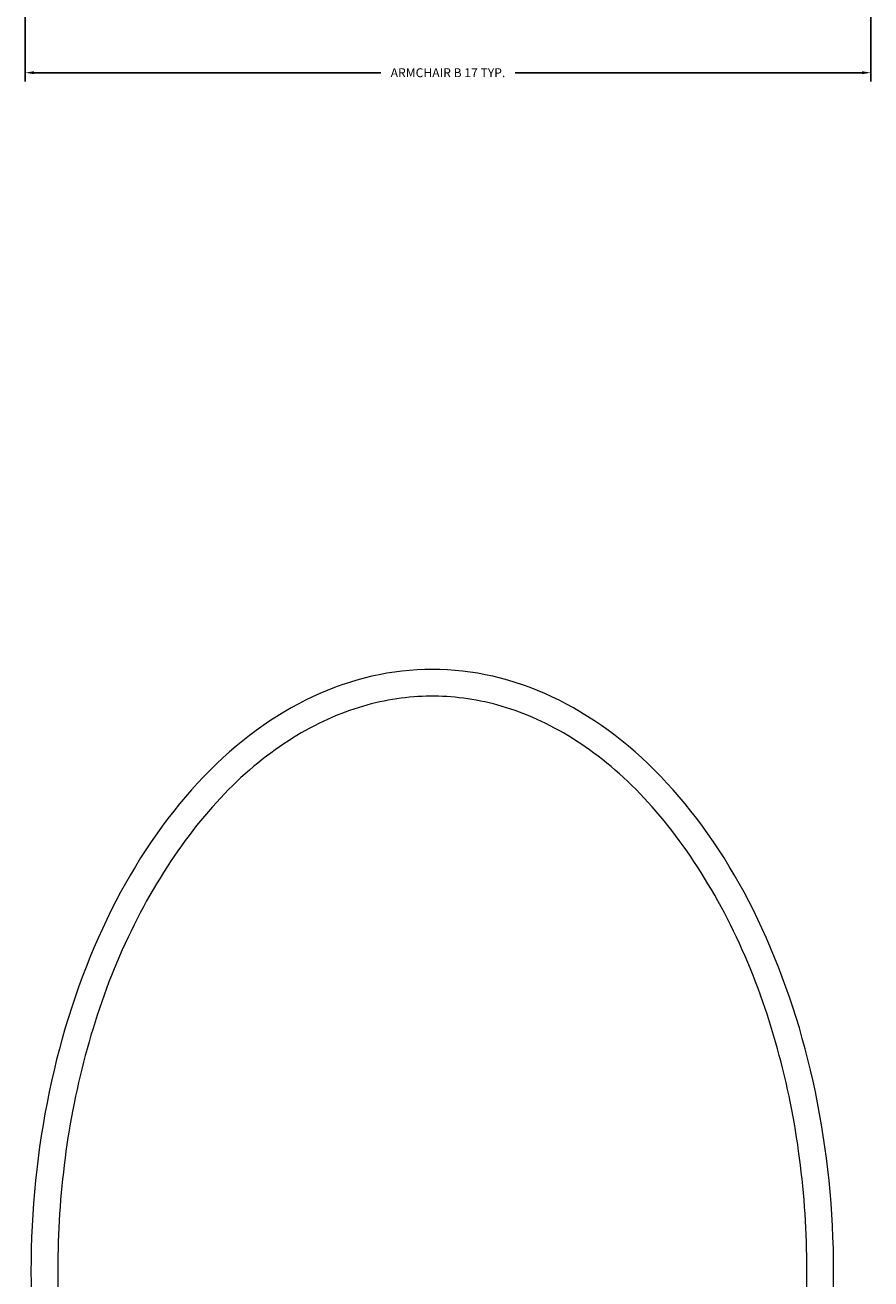
# Model space of a CAD drawing. Units: inches. Extents: x 963 to 2075, y 289 to 2657.
# Tile 75 of 98: x 1467 to 1485, y 2265 to 2290. Entities that reach past the tile are written whole.
import ezdxf

# ---------------------------------------------------------------- set-up
doc = ezdxf.new("R2010")
doc.units = ezdxf.units.IN
doc.layers.add('A-ANNO-DIMS', color=2, linetype='Continuous', lineweight=18)
doc.layers.add('A-FURN', color=8, linetype='Continuous', lineweight=18)
doc.styles.get("Standard").update_dxf_attribs({"font": 'arial.ttf'})
doc.dimstyles.get("Standard").update_dxf_attribs({"dimtxt": 0.18, "dimasz": 0.18, "dimexe": 0.18, "dimexo": 0.0625, "dimgap": 0.09, "dimtad": 0, "dimtih": 1, "dimtoh": 1, "dimdec": 4, "dimzin": 0, "dimdsep": 46, "dimtxsty": 'Standard', "dimcen": 0.09, "dimadec": 0, "dimazin": 0, "dimtfac": 1, "dimtdec": 4, "dimtofl": 0, "dimtmove": 0, "dimatfit": 3, "dimfxl": 1, "dimtolj": 1, "dimtzin": 0, "dimarcsym": 0})

# ---------------------------------------------------------------- blocks, each defined once
blk = doc.blocks.new('TABLE-OVAL')
at = {"ltscale": 0.03}
blk.add_polyline3d([(7.656, -0.197, 0), (7.809, -0.194, 0), (7.963, -0.188, 0), (8.116, -0.177, 0), (8.269, -0.162, 0), (8.422, -0.142, 0), (8.575, -0.118, 0), (8.727, -0.09, 0), (8.879, -0.057, 0), (9.031, -0.021, 0), (9.182, 0.021, 0), (9.332, 0.066, 0), (9.482, 0.116, 0), (9.632, 0.17, 0), (9.78, 0.228, 0), (9.928, 0.29, 0), (10.075, 0.357, 0), (10.221, 0.428, 0), (10.366, 0.503, 0), (10.51, 0.582, 0), (10.653, 0.665, 0), (10.796, 0.752, 0), (10.937, 0.843, 0), (11.076, 0.938, 0), (11.215, 1.037, 0), (11.352, 1.14, 0), (11.488, 1.247, 0), (11.623, 1.358, 0), (11.756, 1.472, 0), (11.888, 1.59, 0), (12.018, 1.712, 0), (12.147, 1.838, 0), (12.274, 1.967, 0), (12.399, 2.1, 0), (12.523, 2.237, 0), (12.645, 2.376, 0), (12.765, 2.52, 0), (12.883, 2.666, 0), (13, 2.817, 0), (13.114, 2.97, 0), (13.227, 3.126, 0), (13.337, 3.286, 0), (13.446, 3.449, 0), (13.552, 3.615, 0), (13.657, 3.784, 0), (13.759, 3.955, 0), (13.859, 4.13, 0), (13.957, 4.308, 0), (14.052, 4.488, 0), (14.145, 4.671, 0), (14.236, 4.856, 0), (14.325, 5.044, 0), (14.411, 5.235, 0), (14.495, 5.428, 0), (14.576, 5.623, 0), (14.655, 5.821, 0), (14.731, 6.021, 0), (14.805, 6.222, 0), (14.877, 6.426, 0), (14.945, 6.632, 0), (15.011, 6.84, 0), (15.075, 7.05, 0), (15.135, 7.261, 0), (15.193, 7.475, 0), (15.249, 7.689, 0), (15.301, 7.906, 0), (15.351, 8.123, 0), (15.399, 8.343, 0), (15.443, 8.563, 0), (15.485, 8.785, 0), (15.523, 9.007, 0), (15.559, 9.231, 0), (15.592, 9.456, 0), (15.623, 9.682, 0), (15.65, 9.908, 0), (15.675, 10.136, 0), (15.697, 10.364, 0), (15.715, 10.592, 0), (15.731, 10.821, 0), (15.744, 11.051, 0), (15.755, 11.28, 0), (15.762, 11.51, 0), (15.766, 11.741, 0), (15.768, 11.971, 0), (15.766, 12.201, 0), (15.762, 12.431, 0), (15.755, 12.661, 0), (15.744, 12.891, 0), (15.731, 13.12, 0), (15.715, 13.349, 0), (15.697, 13.578, 0), (15.675, 13.806, 0), (15.65, 14.033, 0), (15.623, 14.26, 0), (15.592, 14.486, 0), (15.559, 14.71, 0), (15.523, 14.934, 0), (15.485, 15.157, 0), (15.443, 15.379, 0), (15.399, 15.599, 0), (15.351, 15.818, 0), (15.301, 16.036, 0), (15.249, 16.252, 0), (15.193, 16.467, 0), (15.135, 16.68, 0), (15.075, 16.892, 0), (15.011, 17.101, 0), (14.945, 17.309, 0), (14.877, 17.515, 0), (14.805, 17.719, 0), (14.731, 17.921, 0), (14.655, 18.121, 0), (14.576, 18.318, 0), (14.495, 18.514, 0), (14.411, 18.707, 0), (14.325, 18.897, 0), (14.236, 19.085, 0), (14.145, 19.271, 0), (14.052, 19.454, 0), (13.957, 19.634, 0), (13.859, 19.811, 0), (13.759, 19.986, 0), (13.657, 20.158, 0), (13.552, 20.327, 0), (13.446, 20.493, 0), (13.337, 20.656, 0), (13.227, 20.815, 0), (13.114, 20.972, 0), (13, 21.125, 0), (12.883, 21.275, 0), (12.765, 21.422, 0), (12.645, 21.565, 0), (12.523, 21.705, 0), (12.399, 21.842, 0), (12.274, 21.974, 0), (12.147, 22.104, 0), (12.018, 22.229, 0), (11.888, 22.351, 0), (11.756, 22.47, 0), (11.623, 22.584, 0), (11.488, 22.695, 0), (11.352, 22.802, 0), (11.215, 22.905, 0), (11.076, 23.004, 0), (10.937, 23.099, 0), (10.796, 23.19, 0), (10.653, 23.277, 0), (10.51, 23.36, 0), (10.366, 23.439, 0), (10.221, 23.514, 0), (10.075, 23.585, 0), (9.928, 23.651, 0), (9.78, 23.714, 0), (9.632, 23.772, 0), (9.482, 23.826, 0), (9.332, 23.876, 0), (9.182, 23.921, 0), (9.031, 23.962, 0), (8.879, 23.999, 0), (8.727, 24.032, 0), (8.575, 24.06, 0), (8.422, 24.084, 0), (8.269, 24.103, 0), (8.116, 24.119, 0), (7.963, 24.13, 0), (7.809, 24.136, 0), (7.656, 24.138, 0), (7.502, 24.136, 0), (7.349, 24.13, 0), (7.196, 24.119, 0), (7.042, 24.103, 0), (6.89, 24.084, 0), (6.737, 24.06, 0), (6.585, 24.032, 0), (6.433, 23.999, 0), (6.281, 23.962, 0), (6.13, 23.921, 0), (5.979, 23.876, 0), (5.83, 23.826, 0), (5.68, 23.772, 0), (5.532, 23.714, 0), (5.384, 23.651, 0), (5.237, 23.585, 0), (5.091, 23.514, 0), (4.946, 23.439, 0), (4.802, 23.36, 0), (4.658, 23.277, 0), (4.516, 23.19, 0), (4.375, 23.099, 0), (4.236, 23.004, 0), (4.097, 22.905, 0), (3.96, 22.802, 0), (3.824, 22.695, 0), (3.689, 22.584, 0), (3.556, 22.47, 0), (3.424, 22.351, 0), (3.294, 22.229, 0), (3.165, 22.104, 0), (3.038, 21.974, 0), (2.913, 21.842, 0), (2.789, 21.705, 0), (2.667, 21.565, 0), (2.547, 21.422, 0), (2.429, 21.275, 0), (2.312, 21.125, 0), (2.198, 20.972, 0), (2.085, 20.815, 0), (1.975, 20.656, 0), (1.866, 20.493, 0), (1.76, 20.327, 0), (1.655, 20.158, 0), (1.553, 19.986, 0), (1.453, 19.811, 0), (1.355, 19.634, 0), (1.26, 19.454, 0), (1.166, 19.271, 0), (1.076, 19.085, 0), (0.987, 18.897, 0), (0.901, 18.707, 0), (0.817, 18.514, 0), (0.736, 18.318, 0), (0.657, 18.121, 0), (0.58, 17.921, 0), (0.507, 17.719, 0), (0.435, 17.515, 0), (0.367, 17.309, 0), (0.301, 17.101, 0), (0.237, 16.892, 0), (0.177, 16.68, 0), (0.118, 16.467, 0), (0.063, 16.252, 0), (0.01, 16.036, 0), (-0.039, 15.818, 0), (-0.087, 15.599, 0), (-0.131, 15.379, 0), (-0.173, 15.157, 0), (-0.211, 14.934, 0), (-0.247, 14.71, 0), (-0.281, 14.486, 0), (-0.311, 14.26, 0), (-0.338, 14.033, 0), (-0.363, 13.806, 0), (-0.385, 13.578, 0), (-0.403, 13.349, 0), (-0.419, 13.12, 0), (-0.432, 12.891, 0), (-0.443, 12.661, 0), (-0.45, 12.431, 0), (-0.454, 12.201, 0), (-0.456, 11.971, 0), (-0.454, 11.741, 0), (-0.45, 11.51, 0), (-0.443, 11.28, 0), (-0.432, 11.051, 0), (-0.419, 10.821, 0), (-0.403, 10.592, 0), (-0.385, 10.364, 0), (-0.363, 10.136, 0), (-0.338, 9.908, 0), (-0.311, 9.682, 0), (-0.281, 9.456, 0), (-0.247, 9.231, 0), (-0.211, 9.007, 0), (-0.173, 8.785, 0), (-0.131, 8.563, 0), (-0.087, 8.343, 0), (-0.039, 8.123, 0), (0.01, 7.906, 0), (0.063, 7.689, 0), (0.118, 7.475, 0), (0.177, 7.261, 0), (0.237, 7.05, 0), (0.301, 6.84, 0), (0.367, 6.632, 0), (0.435, 6.426, 0), (0.507, 6.222, 0), (0.58, 6.021, 0), (0.657, 5.821, 0), (0.736, 5.623, 0), (0.817, 5.428, 0), (0.901, 5.235, 0), (0.987, 5.044, 0), (1.076, 4.856, 0), (1.166, 4.671, 0), (1.26, 4.488, 0), (1.355, 4.308, 0), (1.453, 4.13, 0), (1.553, 3.955, 0), (1.655, 3.784, 0), (1.76, 3.615, 0), (1.866, 3.449, 0), (1.975, 3.286, 0), (2.085, 3.126, 0), (2.198, 2.97, 0), (2.312, 2.817, 0), (2.429, 2.666, 0), (2.547, 2.52, 0), (2.667, 2.376, 0), (2.789, 2.237, 0), (2.913, 2.1, 0), (3.038, 1.967, 0), (3.165, 1.838, 0), (3.294, 1.712, 0), (3.424, 1.59, 0), (3.556, 1.472, 0), (3.689, 1.358, 0), (3.824, 1.247, 0), (3.96, 1.14, 0), (4.097, 1.037, 0), (4.236, 0.938, 0), (4.375, 0.843, 0), (4.516, 0.752, 0), (4.658, 0.665, 0), (4.802, 0.582, 0), (4.946, 0.503, 0), (5.091, 0.428, 0), (5.237, 0.357, 0), (5.384, 0.29, 0), (5.532, 0.228, 0), (5.68, 0.17, 0), (5.83, 0.116, 0), (5.979, 0.066, 0), (6.13, 0.021, 0), (6.281, -0.021, 0), (6.433, -0.057, 0), (6.585, -0.09, 0), (6.737, -0.118, 0), (6.89, -0.142, 0), (7.042, -0.162, 0), (7.196, -0.177, 0), (7.349, -0.188, 0), (7.502, -0.194, 0), (7.656, -0.197, 0)], dxfattribs=at)
blk.add_polyline3d([(7.656, 0.344, 0), (7.739, 0.345, 0), (7.822, 0.347, 0), (7.906, 0.351, 0), (7.99, 0.356, 0), (8.074, 0.362, 0), (8.159, 0.37, 0), (8.244, 0.38, 0), (8.33, 0.391, 0), (8.415, 0.404, 0), (8.501, 0.418, 0), (8.588, 0.434, 0), (8.674, 0.451, 0), (8.761, 0.47, 0), (8.848, 0.491, 0), (8.935, 0.513, 0), (9.023, 0.538, 0), (9.11, 0.563, 0), (9.198, 0.591, 0), (9.286, 0.62, 0), (9.375, 0.651, 0), (9.463, 0.684, 0), (9.552, 0.719, 0), (9.64, 0.755, 0), (9.729, 0.794, 0), (9.818, 0.834, 0), (9.907, 0.876, 0), (9.995, 0.92, 0), (10.084, 0.966, 0), (10.173, 1.013, 0), (10.262, 1.063, 0), (10.35, 1.114, 0), (10.439, 1.167, 0), (10.527, 1.222, 0), (10.615, 1.279, 0), (10.703, 1.338, 0), (10.791, 1.398, 0), (10.878, 1.461, 0), (10.965, 1.525, 0), (11.052, 1.592, 0), (11.139, 1.66, 0), (11.225, 1.73, 0), (11.311, 1.802, 0), (11.396, 1.876, 0), (11.481, 1.952, 0), (11.565, 2.03, 0), (11.649, 2.109, 0), (11.733, 2.191, 0), (11.815, 2.275, 0), (11.898, 2.361, 0), (11.98, 2.448, 0), (12.061, 2.537, 0), (12.141, 2.629, 0), (12.221, 2.721, 0), (12.301, 2.816, 0), (12.379, 2.912, 0), (12.457, 3.01, 0), (12.535, 3.11, 0), (12.611, 3.211, 0), (12.687, 3.314, 0), (12.762, 3.418, 0), (12.836, 3.524, 0), (12.909, 3.632, 0), (12.982, 3.741, 0), (13.053, 3.851, 0), (13.124, 3.963, 0), (13.194, 4.076, 0), (13.262, 4.191, 0), (13.33, 4.307, 0), (13.397, 4.424, 0), (13.463, 4.543, 0), (13.528, 4.662, 0), (13.591, 4.783, 0), (13.654, 4.906, 0), (13.716, 5.029, 0), (13.776, 5.154, 0), (13.835, 5.279, 0), (13.893, 5.406, 0), (13.95, 5.534, 0), (14.006, 5.663, 0), (14.061, 5.792, 0), (14.114, 5.923, 0), (14.166, 6.055, 0), (14.217, 6.188, 0), (14.266, 6.321, 0), (14.314, 6.455, 0), (14.361, 6.589, 0), (14.406, 6.723, 0), (14.45, 6.858, 0), (14.493, 6.993, 0), (14.535, 7.129, 0), (14.575, 7.265, 0), (14.614, 7.401, 0), (14.652, 7.537, 0), (14.688, 7.674, 0), (14.724, 7.811, 0), (14.758, 7.948, 0), (14.791, 8.086, 0), (14.822, 8.223, 0), (14.852, 8.361, 0), (14.882, 8.5, 0), (14.909, 8.638, 0), (14.936, 8.777, 0), (14.961, 8.916, 0), (14.986, 9.055, 0), (15.009, 9.194, 0), (15.031, 9.334, 0), (15.051, 9.473, 0), (15.071, 9.613, 0), (15.089, 9.753, 0), (15.106, 9.893, 0), (15.122, 10.033, 0), (15.137, 10.174, 0), (15.151, 10.314, 0), (15.163, 10.455, 0), (15.175, 10.596, 0), (15.185, 10.736, 0), (15.194, 10.877, 0), (15.202, 11.018, 0), (15.209, 11.159, 0), (15.215, 11.3, 0), (15.219, 11.441, 0), (15.223, 11.583, 0), (15.225, 11.724, 0), (15.227, 11.865, 0), (15.227, 12.006, 0), (15.226, 12.147, 0), (15.224, 12.288, 0), (15.221, 12.43, 0), (15.217, 12.571, 0), (15.212, 12.712, 0), (15.205, 12.853, 0), (15.198, 12.994, 0), (15.19, 13.135, 0), (15.18, 13.276, 0), (15.169, 13.416, 0), (15.157, 13.557, 0), (15.144, 13.698, 0), (15.13, 13.838, 0), (15.114, 13.978, 0), (15.098, 14.119, 0), (15.08, 14.259, 0), (15.061, 14.399, 0), (15.041, 14.538, 0), (15.02, 14.678, 0), (14.997, 14.817, 0), (14.974, 14.956, 0), (14.949, 15.095, 0), (14.923, 15.234, 0), (14.896, 15.373, 0), (14.867, 15.511, 0), (14.837, 15.649, 0), (14.806, 15.787, 0), (14.774, 15.925, 0), (14.741, 16.062, 0), (14.706, 16.199, 0), (14.67, 16.336, 0), (14.633, 16.473, 0), (14.595, 16.609, 0), (14.555, 16.745, 0), (14.514, 16.881, 0), (14.472, 17.016, 0), (14.428, 17.151, 0), (14.384, 17.286, 0), (14.338, 17.42, 0), (14.29, 17.554, 0), (14.241, 17.687, 0), (14.191, 17.821, 0), (14.14, 17.953, 0), (14.087, 18.084, 0), (14.034, 18.214, 0), (13.978, 18.344, 0), (13.922, 18.472, 0), (13.865, 18.599, 0), (13.806, 18.725, 0), (13.746, 18.85, 0), (13.685, 18.974, 0), (13.623, 19.097, 0), (13.56, 19.219, 0), (13.495, 19.339, 0), (13.43, 19.458, 0), (13.364, 19.576, 0), (13.296, 19.693, 0), (13.228, 19.808, 0), (13.159, 19.922, 0), (13.089, 20.035, 0), (13.017, 20.146, 0), (12.945, 20.255, 0), (12.873, 20.364, 0), (12.799, 20.47, 0), (12.724, 20.576, 0), (12.649, 20.679, 0), (12.573, 20.781, 0), (12.496, 20.882, 0), (12.418, 20.981, 0), (12.34, 21.078, 0), (12.261, 21.173, 0), (12.182, 21.267, 0), (12.101, 21.359, 0), (12.02, 21.449, 0), (11.939, 21.537, 0), (11.857, 21.624, 0), (11.774, 21.709, 0), (11.691, 21.791, 0), (11.607, 21.872, 0), (11.523, 21.951, 0), (11.438, 22.028, 0), (11.353, 22.103, 0), (11.268, 22.176, 0), (11.182, 22.247, 0), (11.095, 22.316, 0), (11.009, 22.383, 0), (10.922, 22.449, 0), (10.835, 22.512, 0), (10.747, 22.574, 0), (10.659, 22.633, 0), (10.571, 22.691, 0), (10.483, 22.747, 0), (10.395, 22.801, 0), (10.306, 22.854, 0), (10.217, 22.904, 0), (10.129, 22.952, 0), (10.04, 22.999, 0), (9.951, 23.044, 0), (9.862, 23.087, 0), (9.773, 23.128, 0), (9.685, 23.167, 0), (9.596, 23.205, 0), (9.507, 23.24, 0), (9.419, 23.274, 0), (9.331, 23.306, 0), (9.242, 23.336, 0), (9.154, 23.365, 0), (9.067, 23.391, 0), (8.979, 23.416, 0), (8.892, 23.44, 0), (8.804, 23.461, 0), (8.718, 23.481, 0), (8.631, 23.499, 0), (8.544, 23.516, 0), (8.458, 23.531, 0), (8.373, 23.545, 0), (8.287, 23.557, 0), (8.202, 23.567, 0), (8.117, 23.576, 0), (8.032, 23.583, 0), (7.948, 23.589, 0), (7.864, 23.593, 0), (7.781, 23.596, 0), (7.697, 23.597, 0), (7.615, 23.597, 0), (7.531, 23.596, 0), (7.448, 23.593, 0), (7.364, 23.589, 0), (7.28, 23.583, 0), (7.195, 23.576, 0), (7.11, 23.567, 0), (7.025, 23.557, 0), (6.939, 23.545, 0), (6.854, 23.531, 0), (6.767, 23.516, 0), (6.681, 23.499, 0), (6.594, 23.481, 0), (6.507, 23.461, 0), (6.42, 23.44, 0), (6.333, 23.416, 0), (6.245, 23.391, 0), (6.158, 23.365, 0), (6.07, 23.336, 0), (5.981, 23.306, 0), (5.893, 23.274, 0), (5.805, 23.24, 0), (5.716, 23.205, 0), (5.627, 23.167, 0), (5.539, 23.128, 0), (5.45, 23.087, 0), (5.361, 23.044, 0), (5.272, 22.999, 0), (5.183, 22.952, 0), (5.095, 22.904, 0), (5.006, 22.854, 0), (4.917, 22.801, 0), (4.829, 22.747, 0), (4.741, 22.691, 0), (4.653, 22.633, 0), (4.565, 22.574, 0), (4.477, 22.512, 0), (4.39, 22.449, 0), (4.303, 22.383, 0), (4.216, 22.316, 0), (4.13, 22.247, 0), (4.044, 22.176, 0), (3.959, 22.103, 0), (3.874, 22.028, 0), (3.789, 21.951, 0), (3.705, 21.872, 0), (3.621, 21.791, 0), (3.538, 21.709, 0), (3.455, 21.624, 0), (3.373, 21.537, 0), (3.292, 21.449, 0), (3.211, 21.359, 0), (3.13, 21.267, 0), (3.051, 21.173, 0), (2.972, 21.078, 0), (2.893, 20.981, 0), (2.816, 20.882, 0), (2.739, 20.781, 0), (2.663, 20.679, 0), (2.588, 20.576, 0), (2.513, 20.47, 0), (2.439, 20.364, 0), (2.366, 20.255, 0), (2.294, 20.146, 0), (2.223, 20.035, 0), (2.153, 19.922, 0), (2.084, 19.808, 0), (2.016, 19.693, 0), (1.948, 19.576, 0), (1.882, 19.458, 0), (1.817, 19.339, 0), (1.752, 19.219, 0), (1.689, 19.097, 0), (1.627, 18.974, 0), (1.566, 18.85, 0), (1.506, 18.725, 0), (1.447, 18.599, 0), (1.39, 18.472, 0), (1.334, 18.344, 0), (1.278, 18.214, 0), (1.225, 18.084, 0), (1.172, 17.953, 0), (1.121, 17.821, 0), (1.071, 17.687, 0), (1.022, 17.554, 0), (0.974, 17.42, 0), (0.928, 17.286, 0), (0.884, 17.151, 0), (0.84, 17.016, 0), (0.798, 16.881, 0), (0.757, 16.745, 0), (0.717, 16.609, 0), (0.679, 16.473, 0), (0.642, 16.336, 0), (0.606, 16.199, 0), (0.571, 16.062, 0), (0.538, 15.925, 0), (0.505, 15.787, 0), (0.475, 15.649, 0), (0.445, 15.511, 0), (0.416, 15.373, 0), (0.389, 15.234, 0), (0.363, 15.095, 0), (0.338, 14.956, 0), (0.315, 14.817, 0), (0.292, 14.678, 0), (0.271, 14.538, 0), (0.251, 14.399, 0), (0.232, 14.259, 0), (0.214, 14.119, 0), (0.198, 13.978, 0), (0.182, 13.838, 0), (0.168, 13.698, 0), (0.155, 13.557, 0), (0.143, 13.416, 0), (0.132, 13.276, 0), (0.122, 13.135, 0), (0.114, 12.994, 0), (0.106, 12.853, 0), (0.1, 12.712, 0), (0.095, 12.571, 0), (0.091, 12.43, 0), (0.088, 12.288, 0), (0.086, 12.147, 0), (0.085, 12.006, 0), (0.085, 11.865, 0), (0.087, 11.724, 0), (0.089, 11.583, 0), (0.093, 11.441, 0), (0.097, 11.3, 0), (0.103, 11.159, 0), (0.11, 11.018, 0), (0.118, 10.877, 0), (0.127, 10.736, 0), (0.137, 10.596, 0), (0.149, 10.455, 0), (0.161, 10.314, 0), (0.175, 10.174, 0), (0.19, 10.033, 0), (0.206, 9.893, 0), (0.223, 9.753, 0), (0.241, 9.613, 0), (0.261, 9.473, 0), (0.281, 9.334, 0), (0.303, 9.194, 0), (0.326, 9.055, 0), (0.35, 8.916, 0), (0.376, 8.777, 0), (0.403, 8.638, 0), (0.43, 8.5, 0), (0.46, 8.361, 0), (0.49, 8.223, 0), (0.521, 8.086, 0), (0.554, 7.948, 0), (0.588, 7.811, 0), (0.623, 7.674, 0), (0.66, 7.537, 0), (0.698, 7.401, 0), (0.737, 7.265, 0), (0.777, 7.129, 0), (0.819, 6.993, 0), (0.862, 6.858, 0), (0.906, 6.723, 0), (0.951, 6.589, 0), (0.998, 6.455, 0), (1.046, 6.321, 0), (1.095, 6.188, 0), (1.146, 6.055, 0), (1.198, 5.923, 0), (1.251, 5.792, 0), (1.306, 5.663, 0), (1.362, 5.534, 0), (1.418, 5.406, 0), (1.477, 5.279, 0), (1.536, 5.154, 0), (1.596, 5.029, 0), (1.658, 4.906, 0), (1.721, 4.783, 0), (1.784, 4.662, 0), (1.849, 4.543, 0), (1.915, 4.424, 0), (1.982, 4.307, 0), (2.05, 4.191, 0), (2.118, 4.076, 0), (2.188, 3.963, 0), (2.259, 3.851, 0), (2.33, 3.741, 0), (2.403, 3.632, 0), (2.476, 3.524, 0), (2.55, 3.418, 0), (2.625, 3.314, 0), (2.701, 3.211, 0), (2.777, 3.11, 0), (2.855, 3.01, 0), (2.933, 2.912, 0), (3.011, 2.816, 0), (3.09, 2.721, 0), (3.17, 2.629, 0), (3.251, 2.537, 0), (3.332, 2.448, 0), (3.414, 2.361, 0), (3.497, 2.275, 0), (3.579, 2.191, 0), (3.663, 2.109, 0), (3.747, 2.03, 0), (3.831, 1.952, 0), (3.916, 1.876, 0), (4.001, 1.802, 0), (4.087, 1.73, 0), (4.173, 1.66, 0), (4.26, 1.592, 0), (4.347, 1.525, 0), (4.434, 1.461, 0), (4.521, 1.398, 0), (4.609, 1.338, 0), (4.697, 1.279, 0), (4.785, 1.222, 0), (4.873, 1.167, 0), (4.962, 1.114, 0), (5.05, 1.063, 0), (5.139, 1.013, 0), (5.228, 0.966, 0), (5.316, 0.92, 0), (5.405, 0.876, 0), (5.494, 0.834, 0), (5.583, 0.794, 0), (5.672, 0.755, 0), (5.76, 0.719, 0), (5.849, 0.684, 0), (5.937, 0.651, 0), (6.026, 0.62, 0), (6.114, 0.591, 0), (6.201, 0.563, 0), (6.289, 0.538, 0), (6.377, 0.513, 0), (6.464, 0.491, 0), (6.551, 0.47, 0), (6.638, 0.451, 0), (6.724, 0.434, 0), (6.811, 0.418, 0), (6.897, 0.404, 0), (6.982, 0.391, 0), (7.068, 0.38, 0), (7.153, 0.37, 0), (7.237, 0.362, 0), (7.322, 0.356, 0), (7.406, 0.351, 0), (7.49, 0.347, 0), (7.573, 0.345, 0), (7.656, 0.344, 0)])
blk = doc.blocks.new('*D24')
at = {"layer": 'A-ANNO-DIMS', "color": 0, "lineweight": -2, "transparency": 16777216}
for p, q in [((1467.425, 2291.701), (1467.425, 2289.019)), ((1484.522, 2291.701), (1484.522, 2289.019)), ((1467.605, 2289.199), (1474.616, 2289.199)), ((1484.342, 2289.199), (1477.331, 2289.199))]:
    blk.add_line(p, q, dxfattribs=at)
at = {"layer": 'A-ANNO-DIMS', "color": 0, "transparency": 16777216}
for points in [[(1467.605, 2289.229), (1467.605, 2289.169), (1467.425, 2289.199)], [(1484.342, 2289.229), (1484.342, 2289.169), (1484.522, 2289.199)]]:
    blk.add_solid(points, dxfattribs=at)
at = {"layer": 'Defpoints', "color": 0, "transparency": 16777216}
for p in [(1467.425, 2291.764), (1484.522, 2291.764), (1484.522, 2289.199)]:
    blk.add_point(p, dxfattribs=at)
at = {"layer": 'A-ANNO-DIMS', "color": 0, "transparency": 16777216, "insert": (1475.973, 2289.199), "char_height": 0.18, "attachment_point": 5}
blk.add_mtext('\\A1;ARMCHAIR B 17 TYP.', dxfattribs=at)

msp = doc.modelspace()

# ---------------------------------------------------------------- block references
at = {"layer": 'A-FURN'}
msp.add_blockref('TABLE-OVAL', (1468, 2253), dxfattribs=at)

# ---------------------------------------------------------------- dimensions: what is measured, and where the dimension line sits
at = {"layer": 'A-ANNO-DIMS'}
dim = msp.add_linear_dim(base=(1484.522, 2289.199), p1=(1467.425, 2291.764), p2=(1484.522, 2291.764), text='ARMCHAIR B <> TYP.', dimstyle='Standard', override={"dimdec": 0, "dimlfac": 1, "dimrnd": 0, "dimzin": 0, "dimdsep": 46, "dimlunit": 2}, dxfattribs=at)
dim.commit()
dim.dimension.update_dxf_attribs({"geometry": '*D24', "text_midpoint": (1475.973, 2289.199)})

doc.saveas('drawing.dxf')
